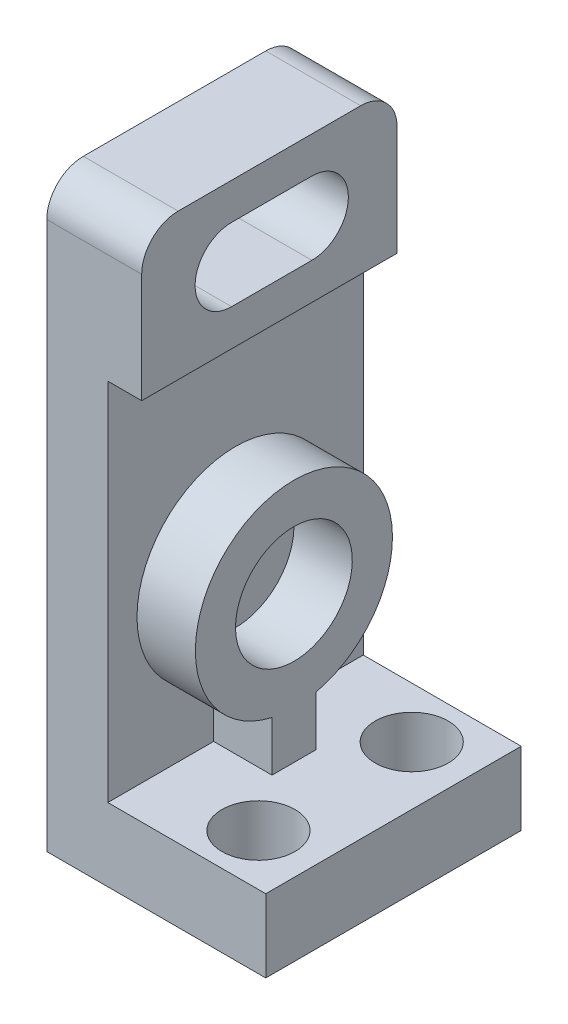
ISO-10303-21;
HEADER;
FILE_DESCRIPTION(('STEP AP214'),'2;1');
FILE_NAME('part.step','',(''),(''),'','','');
FILE_SCHEMA(('AUTOMOTIVE_DESIGN { 1 0 10303 214 1 1 1 1 }'));
ENDSEC;
DATA;
#1=APPLICATION_CONTEXT('core data for automotive mechanical design processes');
#2=APPLICATION_PROTOCOL_DEFINITION('international standard','automotive_design',2000,#1);
#3=PRODUCT_CONTEXT('',#1,'mechanical');
#4=PRODUCT('Part','Part','',(#3));
#5=PRODUCT_RELATED_PRODUCT_CATEGORY('part','',(#4));
#6=PRODUCT_DEFINITION_FORMATION('','',#4);
#7=PRODUCT_DEFINITION_CONTEXT('part definition',#1,'design');
#8=PRODUCT_DEFINITION('design','',#6,#7);
#9=PRODUCT_DEFINITION_SHAPE('','',#8);
#10=(LENGTH_UNIT() NAMED_UNIT(*) SI_UNIT(.MILLI.,.METRE.));
#11=(NAMED_UNIT(*) PLANE_ANGLE_UNIT() SI_UNIT($,.RADIAN.));
#12=(NAMED_UNIT(*) SI_UNIT($,.STERADIAN.) SOLID_ANGLE_UNIT());
#13=UNCERTAINTY_MEASURE_WITH_UNIT(LENGTH_MEASURE(1.E-05),#10,'distance_accuracy_value','');
#14=(GEOMETRIC_REPRESENTATION_CONTEXT(3) GLOBAL_UNCERTAINTY_ASSIGNED_CONTEXT((#13)) GLOBAL_UNIT_ASSIGNED_CONTEXT((#10,
#11,#12)) REPRESENTATION_CONTEXT('',''));
#15=CARTESIAN_POINT('',(0.,0.,0.));
#16=DIRECTION('',(0.,0.,1.));
#17=DIRECTION('',(1.,0.,0.));
#18=AXIS2_PLACEMENT_3D('',#15,#16,#17);
#19=CARTESIAN_POINT('',(8.35866126385831,-30.,-17.5));
#20=DIRECTION('',(0.,-1.,0.));
#21=DIRECTION('',(1.,0.,0.));
#22=AXIS2_PLACEMENT_3D('',#19,#20,#21);
#23=PLANE('',#22);
#24=CARTESIAN_POINT('',(22.,-30.,-10.5));
#25=DIRECTION('',(0.,1.,0.));
#26=DIRECTION('',(-1.,0.,0.));
#27=AXIS2_PLACEMENT_3D('',#24,#25,#26);
#28=CIRCLE('',#27,5.);
#29=CARTESIAN_POINT('',(17.,-30.,-10.5));
#30=VERTEX_POINT('',#29);
#31=EDGE_CURVE('E202',#30,#30,#28,.T.);
#32=ORIENTED_EDGE('',*,*,#31,.F.);
#33=EDGE_LOOP('',(#32));
#34=FACE_BOUND('',#33,.T.);
#35=CARTESIAN_POINT('',(22.,-30.,10.5));
#36=DIRECTION('',(0.,1.,0.));
#37=DIRECTION('',(1.,0.,0.));
#38=AXIS2_PLACEMENT_3D('',#35,#36,#37);
#39=CIRCLE('',#38,5.);
#40=CARTESIAN_POINT('',(27.,-30.,10.5));
#41=VERTEX_POINT('',#40);
#42=EDGE_CURVE('E206',#41,#41,#39,.T.);
#43=ORIENTED_EDGE('',*,*,#42,.F.);
#44=EDGE_LOOP('',(#43));
#45=FACE_BOUND('',#44,.T.);
#46=DIRECTION('',(-1.,0.,0.));
#47=VECTOR('',#46,1.);
#48=CARTESIAN_POINT('',(16.3586612638583,-30.,-3.00000000000001));
#49=LINE('',#48,#47);
#50=CARTESIAN_POINT('',(16.3586612638583,-30.,-3.00000000000001));
#51=VERTEX_POINT('',#50);
#52=CARTESIAN_POINT('',(8.35866126385831,-30.,-3.00000000000001));
#53=VERTEX_POINT('',#52);
#54=EDGE_CURVE('E229',#51,#53,#49,.T.);
#55=ORIENTED_EDGE('',*,*,#54,.F.);
#56=DIRECTION('',(0.,0.,-1.));
#57=VECTOR('',#56,1.);
#58=CARTESIAN_POINT('',(16.3586612638583,-30.,2.99999999999999));
#59=LINE('',#58,#57);
#60=CARTESIAN_POINT('',(16.3586612638583,-30.,2.99999999999999));
#61=VERTEX_POINT('',#60);
#62=EDGE_CURVE('E226',#61,#51,#59,.T.);
#63=ORIENTED_EDGE('',*,*,#62,.F.);
#64=DIRECTION('',(-1.,0.,0.));
#65=VECTOR('',#64,1.);
#66=CARTESIAN_POINT('',(16.3586612638583,-30.,2.99999999999999));
#67=LINE('',#66,#65);
#68=CARTESIAN_POINT('',(8.35866126385831,-30.,2.99999999999999));
#69=VERTEX_POINT('',#68);
#70=EDGE_CURVE('E238',#61,#69,#67,.T.);
#71=ORIENTED_EDGE('',*,*,#70,.T.);
#72=DIRECTION('',(0.,0.,1.));
#73=VECTOR('',#72,1.);
#74=CARTESIAN_POINT('',(8.35866126385831,-30.,-17.5));
#75=LINE('',#74,#73);
#76=CARTESIAN_POINT('',(8.35866126385831,-30.,17.5));
#77=VERTEX_POINT('',#76);
#78=EDGE_CURVE('E273',#69,#77,#75,.T.);
#79=ORIENTED_EDGE('',*,*,#78,.T.);
#80=DIRECTION('',(1.,0.,0.));
#81=VECTOR('',#80,1.);
#82=CARTESIAN_POINT('',(8.35866126385831,-30.,17.5));
#83=LINE('',#82,#81);
#84=CARTESIAN_POINT('',(30.,-30.,17.5));
#85=VERTEX_POINT('',#84);
#86=EDGE_CURVE('E249',#77,#85,#83,.T.);
#87=ORIENTED_EDGE('',*,*,#86,.T.);
#88=DIRECTION('',(0.,0.,1.));
#89=VECTOR('',#88,1.);
#90=CARTESIAN_POINT('',(30.,-30.,-17.5));
#91=LINE('',#90,#89);
#92=CARTESIAN_POINT('',(30.,-30.,-17.5));
#93=VERTEX_POINT('',#92);
#94=EDGE_CURVE('E270',#93,#85,#91,.T.);
#95=ORIENTED_EDGE('',*,*,#94,.F.);
#96=DIRECTION('',(1.,0.,0.));
#97=VECTOR('',#96,1.);
#98=CARTESIAN_POINT('',(8.35866126385831,-30.,-17.5));
#99=LINE('',#98,#97);
#100=CARTESIAN_POINT('',(8.35866126385831,-30.,-17.5));
#101=VERTEX_POINT('',#100);
#102=EDGE_CURVE('E257',#101,#93,#99,.T.);
#103=ORIENTED_EDGE('',*,*,#102,.F.);
#104=EDGE_CURVE('E275',#101,#53,#75,.T.);
#105=ORIENTED_EDGE('',*,*,#104,.T.);
#106=EDGE_LOOP('',(#55,#63,#71,#79,#87,#95,#103,#105));
#107=FACE_BOUND('',#106,.T.);
#108=ADVANCED_FACE('F39',(#34,#45,#107),#23,.F.);
#109=CARTESIAN_POINT('',(8.3586612638583,20.,-17.5));
#110=DIRECTION('',(-1.,0.,0.));
#111=DIRECTION('',(0.,-1.,0.));
#112=AXIS2_PLACEMENT_3D('',#109,#110,#111);
#113=PLANE('',#112);
#114=DIRECTION('',(0.,1.,0.));
#115=VECTOR('',#114,1.);
#116=CARTESIAN_POINT('',(8.35866126385831,-30.,-3.00000000000001));
#117=LINE('',#116,#115);
#118=CARTESIAN_POINT('',(8.35866126385831,-23.1624465810882,-3.00000000000001));
#119=VERTEX_POINT('',#118);
#120=EDGE_CURVE('E217',#53,#119,#117,.T.);
#121=ORIENTED_EDGE('',*,*,#120,.F.);
#122=ORIENTED_EDGE('',*,*,#104,.F.);
#123=DIRECTION('',(0.,-1.,0.));
#124=VECTOR('',#123,1.);
#125=CARTESIAN_POINT('',(8.3586612638583,20.,-17.5));
#126=LINE('',#125,#124);
#127=CARTESIAN_POINT('',(8.3586612638583,20.,-17.5));
#128=VERTEX_POINT('',#127);
#129=EDGE_CURVE('E254',#128,#101,#126,.T.);
#130=ORIENTED_EDGE('',*,*,#129,.F.);
#131=DIRECTION('',(0.,0.,1.));
#132=VECTOR('',#131,1.);
#133=CARTESIAN_POINT('',(8.3586612638583,20.,-17.5));
#134=LINE('',#133,#132);
#135=CARTESIAN_POINT('',(8.3586612638583,20.,17.5));
#136=VERTEX_POINT('',#135);
#137=EDGE_CURVE('E277',#128,#136,#134,.T.);
#138=ORIENTED_EDGE('',*,*,#137,.T.);
#139=DIRECTION('',(0.,-1.,0.));
#140=VECTOR('',#139,1.);
#141=CARTESIAN_POINT('',(8.3586612638583,20.,17.5));
#142=LINE('',#141,#140);
#143=EDGE_CURVE('E261',#136,#77,#142,.T.);
#144=ORIENTED_EDGE('',*,*,#143,.T.);
#145=ORIENTED_EDGE('',*,*,#78,.F.);
#146=DIRECTION('',(0.,1.,0.));
#147=VECTOR('',#146,1.);
#148=CARTESIAN_POINT('',(8.35866126385831,-30.,2.99999999999999));
#149=LINE('',#148,#147);
#150=CARTESIAN_POINT('',(8.35866126385831,-23.1624465810882,2.99999999999999));
#151=VERTEX_POINT('',#150);
#152=EDGE_CURVE('E225',#69,#151,#149,.T.);
#153=ORIENTED_EDGE('',*,*,#152,.T.);
#154=CARTESIAN_POINT('',(8.35866126385831,-10.,0.));
#155=DIRECTION('',(1.,0.,0.));
#156=DIRECTION('',(0.,1.,0.));
#157=AXIS2_PLACEMENT_3D('',#154,#155,#156);
#158=CIRCLE('',#157,13.5);
#159=EDGE_CURVE('E231',#119,#151,#158,.T.);
#160=ORIENTED_EDGE('',*,*,#159,.F.);
#161=EDGE_LOOP('',(#121,#122,#130,#138,#144,#145,#153,#160));
#162=FACE_BOUND('',#161,.T.);
#163=ADVANCED_FACE('F356',(#162),#113,.F.);
#164=CARTESIAN_POINT('',(30.,40.,-17.5));
#165=DIRECTION('',(0.,0.,1.));
#166=DIRECTION('',(0.,-1.,0.));
#167=AXIS2_PLACEMENT_3D('',#164,#165,#166);
#168=PLANE('',#167);
#169=DIRECTION('',(0.,1.,0.));
#170=VECTOR('',#169,1.);
#171=CARTESIAN_POINT('',(0.,40.,-17.5));
#172=LINE('',#171,#170);
#173=CARTESIAN_POINT('',(0.,-40.,-17.5));
#174=VERTEX_POINT('',#173);
#175=CARTESIAN_POINT('',(0.,35.,-17.5));
#176=VERTEX_POINT('',#175);
#177=EDGE_CURVE('E272',#174,#176,#172,.T.);
#178=ORIENTED_EDGE('',*,*,#177,.T.);
#179=DIRECTION('',(-1.,0.,0.));
#180=VECTOR('',#179,1.);
#181=CARTESIAN_POINT('',(30.,35.,-17.5));
#182=LINE('',#181,#180);
#183=CARTESIAN_POINT('',(13.,35.,-17.5));
#184=VERTEX_POINT('',#183);
#185=EDGE_CURVE('E313',#176,#184,#182,.F.);
#186=ORIENTED_EDGE('',*,*,#185,.T.);
#187=DIRECTION('',(0.,-1.,0.));
#188=VECTOR('',#187,1.);
#189=CARTESIAN_POINT('',(13.,40.,-17.5));
#190=LINE('',#189,#188);
#191=CARTESIAN_POINT('',(13.,20.,-17.5));
#192=VERTEX_POINT('',#191);
#193=EDGE_CURVE('E250',#184,#192,#190,.T.);
#194=ORIENTED_EDGE('',*,*,#193,.T.);
#195=DIRECTION('',(-1.,0.,0.));
#196=VECTOR('',#195,1.);
#197=CARTESIAN_POINT('',(13.,20.,-17.5));
#198=LINE('',#197,#196);
#199=EDGE_CURVE('E248',#192,#128,#198,.T.);
#200=ORIENTED_EDGE('',*,*,#199,.T.);
#201=ORIENTED_EDGE('',*,*,#129,.T.);
#202=ORIENTED_EDGE('',*,*,#102,.T.);
#203=DIRECTION('',(0.,1.,0.));
#204=VECTOR('',#203,1.);
#205=CARTESIAN_POINT('',(30.,40.,-17.5));
#206=LINE('',#205,#204);
#207=CARTESIAN_POINT('',(30.,-40.,-17.5));
#208=VERTEX_POINT('',#207);
#209=EDGE_CURVE('E284',#208,#93,#206,.T.);
#210=ORIENTED_EDGE('',*,*,#209,.F.);
#211=DIRECTION('',(-1.,0.,0.));
#212=VECTOR('',#211,1.);
#213=CARTESIAN_POINT('',(30.,-40.,-17.5));
#214=LINE('',#213,#212);
#215=EDGE_CURVE('E293',#208,#174,#214,.T.);
#216=ORIENTED_EDGE('',*,*,#215,.T.);
#217=EDGE_LOOP('',(#178,#186,#194,#200,#201,#202,#210,#216));
#218=FACE_BOUND('',#217,.T.);
#219=ADVANCED_FACE('F332',(#218),#168,.F.);
#220=CARTESIAN_POINT('',(30.,40.,17.5));
#221=DIRECTION('',(0.,-1.,0.));
#222=DIRECTION('',(0.,0.,-1.));
#223=AXIS2_PLACEMENT_3D('',#220,#221,#222);
#224=PLANE('',#223);
#225=DIRECTION('',(0.,0.,1.));
#226=VECTOR('',#225,1.);
#227=CARTESIAN_POINT('',(13.,40.,-17.5));
#228=LINE('',#227,#226);
#229=CARTESIAN_POINT('',(13.,40.,-12.5));
#230=VERTEX_POINT('',#229);
#231=CARTESIAN_POINT('',(13.,40.,12.5));
#232=VERTEX_POINT('',#231);
#233=EDGE_CURVE('E256',#230,#232,#228,.T.);
#234=ORIENTED_EDGE('',*,*,#233,.F.);
#235=DIRECTION('',(-1.,0.,0.));
#236=VECTOR('',#235,1.);
#237=CARTESIAN_POINT('',(30.,40.,-12.5));
#238=LINE('',#237,#236);
#239=CARTESIAN_POINT('',(0.,40.,-12.5));
#240=VERTEX_POINT('',#239);
#241=EDGE_CURVE('E310',#230,#240,#238,.T.);
#242=ORIENTED_EDGE('',*,*,#241,.T.);
#243=DIRECTION('',(0.,0.,1.));
#244=VECTOR('',#243,1.);
#245=CARTESIAN_POINT('',(0.,40.,17.5));
#246=LINE('',#245,#244);
#247=CARTESIAN_POINT('',(0.,40.,12.5));
#248=VERTEX_POINT('',#247);
#249=EDGE_CURVE('E295',#240,#248,#246,.T.);
#250=ORIENTED_EDGE('',*,*,#249,.T.);
#251=DIRECTION('',(-1.,0.,0.));
#252=VECTOR('',#251,1.);
#253=CARTESIAN_POINT('',(30.,40.,12.5));
#254=LINE('',#253,#252);
#255=EDGE_CURVE('E304',#248,#232,#254,.F.);
#256=ORIENTED_EDGE('',*,*,#255,.T.);
#257=EDGE_LOOP('',(#234,#242,#250,#256));
#258=FACE_BOUND('',#257,.T.);
#259=ADVANCED_FACE('F329',(#258),#224,.F.);
#260=CARTESIAN_POINT('',(30.,40.,17.5));
#261=DIRECTION('',(0.,0.,-1.));
#262=DIRECTION('',(0.,1.,0.));
#263=AXIS2_PLACEMENT_3D('',#260,#261,#262);
#264=PLANE('',#263);
#265=DIRECTION('',(0.,-1.,0.));
#266=VECTOR('',#265,1.);
#267=CARTESIAN_POINT('',(13.,40.,17.5));
#268=LINE('',#267,#266);
#269=CARTESIAN_POINT('',(13.,35.,17.5));
#270=VERTEX_POINT('',#269);
#271=CARTESIAN_POINT('',(13.,20.,17.5));
#272=VERTEX_POINT('',#271);
#273=EDGE_CURVE('E246',#270,#272,#268,.T.);
#274=ORIENTED_EDGE('',*,*,#273,.F.);
#275=DIRECTION('',(-1.,0.,0.));
#276=VECTOR('',#275,1.);
#277=CARTESIAN_POINT('',(30.,35.,17.5));
#278=LINE('',#277,#276);
#279=CARTESIAN_POINT('',(0.,35.,17.5));
#280=VERTEX_POINT('',#279);
#281=EDGE_CURVE('E11',#270,#280,#278,.T.);
#282=ORIENTED_EDGE('',*,*,#281,.T.);
#283=DIRECTION('',(0.,-1.,0.));
#284=VECTOR('',#283,1.);
#285=CARTESIAN_POINT('',(0.,40.,17.5));
#286=LINE('',#285,#284);
#287=CARTESIAN_POINT('',(0.,-40.,17.5));
#288=VERTEX_POINT('',#287);
#289=EDGE_CURVE('E300',#280,#288,#286,.T.);
#290=ORIENTED_EDGE('',*,*,#289,.T.);
#291=DIRECTION('',(-1.,0.,0.));
#292=VECTOR('',#291,1.);
#293=CARTESIAN_POINT('',(30.,-40.,17.5));
#294=LINE('',#293,#292);
#295=CARTESIAN_POINT('',(30.,-40.,17.5));
#296=VERTEX_POINT('',#295);
#297=EDGE_CURVE('E305',#296,#288,#294,.T.);
#298=ORIENTED_EDGE('',*,*,#297,.F.);
#299=DIRECTION('',(0.,-1.,0.));
#300=VECTOR('',#299,1.);
#301=CARTESIAN_POINT('',(30.,40.,17.5));
#302=LINE('',#301,#300);
#303=EDGE_CURVE('E289',#85,#296,#302,.T.);
#304=ORIENTED_EDGE('',*,*,#303,.F.);
#305=ORIENTED_EDGE('',*,*,#86,.F.);
#306=ORIENTED_EDGE('',*,*,#143,.F.);
#307=DIRECTION('',(-1.,0.,0.));
#308=VECTOR('',#307,1.);
#309=CARTESIAN_POINT('',(13.,20.,17.5));
#310=LINE('',#309,#308);
#311=EDGE_CURVE('E262',#272,#136,#310,.T.);
#312=ORIENTED_EDGE('',*,*,#311,.F.);
#313=EDGE_LOOP('',(#274,#282,#290,#298,#304,#305,#306,#312));
#314=FACE_BOUND('',#313,.T.);
#315=ADVANCED_FACE('F343',(#314),#264,.F.);
#316=CARTESIAN_POINT('',(30.,-40.,17.5));
#317=DIRECTION('',(0.,1.,0.));
#318=DIRECTION('',(0.,0.,1.));
#319=AXIS2_PLACEMENT_3D('',#316,#317,#318);
#320=PLANE('',#319);
#321=CARTESIAN_POINT('',(22.,-40.,-10.5));
#322=DIRECTION('',(0.,1.,0.));
#323=DIRECTION('',(-1.,0.,0.));
#324=AXIS2_PLACEMENT_3D('',#321,#322,#323);
#325=CIRCLE('',#324,5.);
#326=CARTESIAN_POINT('',(17.,-40.,-10.5));
#327=VERTEX_POINT('',#326);
#328=EDGE_CURVE('E204',#327,#327,#325,.T.);
#329=ORIENTED_EDGE('',*,*,#328,.T.);
#330=EDGE_LOOP('',(#329));
#331=FACE_BOUND('',#330,.T.);
#332=CARTESIAN_POINT('',(22.,-40.,10.5));
#333=DIRECTION('',(0.,1.,0.));
#334=DIRECTION('',(1.,0.,0.));
#335=AXIS2_PLACEMENT_3D('',#332,#333,#334);
#336=CIRCLE('',#335,5.);
#337=CARTESIAN_POINT('',(27.,-40.,10.5));
#338=VERTEX_POINT('',#337);
#339=EDGE_CURVE('E200',#338,#338,#336,.T.);
#340=ORIENTED_EDGE('',*,*,#339,.T.);
#341=EDGE_LOOP('',(#340));
#342=FACE_BOUND('',#341,.T.);
#343=DIRECTION('',(0.,0.,-1.));
#344=VECTOR('',#343,1.);
#345=CARTESIAN_POINT('',(0.,-40.,17.5));
#346=LINE('',#345,#344);
#347=EDGE_CURVE('E286',#288,#174,#346,.T.);
#348=ORIENTED_EDGE('',*,*,#347,.T.);
#349=ORIENTED_EDGE('',*,*,#215,.F.);
#350=DIRECTION('',(0.,0.,-1.));
#351=VECTOR('',#350,1.);
#352=CARTESIAN_POINT('',(30.,-40.,17.5));
#353=LINE('',#352,#351);
#354=EDGE_CURVE('E288',#296,#208,#353,.T.);
#355=ORIENTED_EDGE('',*,*,#354,.F.);
#356=ORIENTED_EDGE('',*,*,#297,.T.);
#357=EDGE_LOOP('',(#348,#349,#355,#356));
#358=FACE_BOUND('',#357,.T.);
#359=ADVANCED_FACE('F338',(#331,#342,#358),#320,.F.);
#360=CARTESIAN_POINT('',(30.,0.,0.));
#361=DIRECTION('',(1.,0.,0.));
#362=DIRECTION('',(0.,0.,-1.));
#363=AXIS2_PLACEMENT_3D('',#360,#361,#362);
#364=PLANE('',#363);
#365=ORIENTED_EDGE('',*,*,#94,.T.);
#366=ORIENTED_EDGE('',*,*,#303,.T.);
#367=ORIENTED_EDGE('',*,*,#354,.T.);
#368=ORIENTED_EDGE('',*,*,#209,.T.);
#369=EDGE_LOOP('',(#365,#366,#367,#368));
#370=FACE_BOUND('',#369,.T.);
#371=ADVANCED_FACE('F361',(#370),#364,.T.);
#372=CARTESIAN_POINT('',(0.,0.,0.));
#373=DIRECTION('',(1.,0.,0.));
#374=DIRECTION('',(0.,0.,-1.));
#375=AXIS2_PLACEMENT_3D('',#372,#373,#374);
#376=PLANE('',#375);
#377=DIRECTION('',(0.,0.,1.));
#378=VECTOR('',#377,1.);
#379=CARTESIAN_POINT('',(0.,35.,5.18095085404985));
#380=LINE('',#379,#378);
#381=CARTESIAN_POINT('',(0.,35.,-5.81904914595015));
#382=VERTEX_POINT('',#381);
#383=CARTESIAN_POINT('',(0.,35.,5.18095085404985));
#384=VERTEX_POINT('',#383);
#385=EDGE_CURVE('E175',#382,#384,#380,.T.);
#386=ORIENTED_EDGE('',*,*,#385,.T.);
#387=CARTESIAN_POINT('',(0.,30.,5.18095085404985));
#388=DIRECTION('',(1.,0.,0.));
#389=DIRECTION('',(0.,1.,0.));
#390=AXIS2_PLACEMENT_3D('',#387,#388,#389);
#391=CIRCLE('',#390,5.);
#392=CARTESIAN_POINT('',(0.,25.,5.18095085404985));
#393=VERTEX_POINT('',#392);
#394=EDGE_CURVE('E168',#384,#393,#391,.T.);
#395=ORIENTED_EDGE('',*,*,#394,.T.);
#396=DIRECTION('',(0.,0.,-1.));
#397=VECTOR('',#396,1.);
#398=CARTESIAN_POINT('',(0.,25.,5.18095085404985));
#399=LINE('',#398,#397);
#400=CARTESIAN_POINT('',(0.,25.,-5.81904914595015));
#401=VERTEX_POINT('',#400);
#402=EDGE_CURVE('E174',#393,#401,#399,.T.);
#403=ORIENTED_EDGE('',*,*,#402,.T.);
#404=CARTESIAN_POINT('',(0.,30.,-5.81904914595015));
#405=DIRECTION('',(1.,0.,0.));
#406=DIRECTION('',(0.,1.,0.));
#407=AXIS2_PLACEMENT_3D('',#404,#405,#406);
#408=CIRCLE('',#407,5.);
#409=EDGE_CURVE('E53',#401,#382,#408,.T.);
#410=ORIENTED_EDGE('',*,*,#409,.T.);
#411=EDGE_LOOP('',(#386,#395,#403,#410));
#412=FACE_BOUND('',#411,.T.);
#413=ORIENTED_EDGE('',*,*,#249,.F.);
#414=CARTESIAN_POINT('',(0.,35.,-12.5));
#415=DIRECTION('',(1.,0.,0.));
#416=DIRECTION('',(0.,0.,-1.));
#417=AXIS2_PLACEMENT_3D('',#414,#415,#416);
#418=CIRCLE('',#417,5.);
#419=EDGE_CURVE('E315',#240,#176,#418,.F.);
#420=ORIENTED_EDGE('',*,*,#419,.T.);
#421=ORIENTED_EDGE('',*,*,#177,.F.);
#422=ORIENTED_EDGE('',*,*,#347,.F.);
#423=ORIENTED_EDGE('',*,*,#289,.F.);
#424=CARTESIAN_POINT('',(0.,35.,12.5));
#425=DIRECTION('',(1.,0.,0.));
#426=DIRECTION('',(0.,0.,-1.));
#427=AXIS2_PLACEMENT_3D('',#424,#425,#426);
#428=CIRCLE('',#427,5.);
#429=EDGE_CURVE('E309',#280,#248,#428,.F.);
#430=ORIENTED_EDGE('',*,*,#429,.T.);
#431=EDGE_LOOP('',(#413,#420,#421,#422,#423,#430));
#432=FACE_BOUND('',#431,.T.);
#433=ADVANCED_FACE('F177',(#412,#432),#376,.F.);
#434=CARTESIAN_POINT('',(13.,20.,-17.5));
#435=DIRECTION('',(0.,1.,0.));
#436=DIRECTION('',(0.,0.,1.));
#437=AXIS2_PLACEMENT_3D('',#434,#435,#436);
#438=PLANE('',#437);
#439=ORIENTED_EDGE('',*,*,#311,.T.);
#440=ORIENTED_EDGE('',*,*,#137,.F.);
#441=ORIENTED_EDGE('',*,*,#199,.F.);
#442=DIRECTION('',(0.,0.,1.));
#443=VECTOR('',#442,1.);
#444=CARTESIAN_POINT('',(13.,20.,-17.5));
#445=LINE('',#444,#443);
#446=EDGE_CURVE('E279',#192,#272,#445,.T.);
#447=ORIENTED_EDGE('',*,*,#446,.T.);
#448=EDGE_LOOP('',(#439,#440,#441,#447));
#449=FACE_BOUND('',#448,.T.);
#450=ADVANCED_FACE('F351',(#449),#438,.F.);
#451=CARTESIAN_POINT('',(13.,40.,-17.5));
#452=DIRECTION('',(-1.,0.,0.));
#453=DIRECTION('',(0.,-1.,0.));
#454=AXIS2_PLACEMENT_3D('',#451,#452,#453);
#455=PLANE('',#454);
#456=DIRECTION('',(0.,0.,-1.));
#457=VECTOR('',#456,1.);
#458=CARTESIAN_POINT('',(13.,25.,5.18095085404985));
#459=LINE('',#458,#457);
#460=CARTESIAN_POINT('',(13.,25.,5.18095085404985));
#461=VERTEX_POINT('',#460);
#462=CARTESIAN_POINT('',(13.,25.,-5.81904914595015));
#463=VERTEX_POINT('',#462);
#464=EDGE_CURVE('E192',#461,#463,#459,.T.);
#465=ORIENTED_EDGE('',*,*,#464,.F.);
#466=CARTESIAN_POINT('',(13.,30.,5.18095085404985));
#467=DIRECTION('',(1.,0.,0.));
#468=DIRECTION('',(0.,1.,0.));
#469=AXIS2_PLACEMENT_3D('',#466,#467,#468);
#470=CIRCLE('',#469,5.);
#471=CARTESIAN_POINT('',(13.,35.,5.18095085404985));
#472=VERTEX_POINT('',#471);
#473=EDGE_CURVE('E65',#472,#461,#470,.T.);
#474=ORIENTED_EDGE('',*,*,#473,.F.);
#475=DIRECTION('',(0.,0.,1.));
#476=VECTOR('',#475,1.);
#477=CARTESIAN_POINT('',(13.,35.,5.18095085404985));
#478=LINE('',#477,#476);
#479=CARTESIAN_POINT('',(13.,35.,-5.81904914595015));
#480=VERTEX_POINT('',#479);
#481=EDGE_CURVE('E185',#480,#472,#478,.T.);
#482=ORIENTED_EDGE('',*,*,#481,.F.);
#483=CARTESIAN_POINT('',(13.,30.,-5.81904914595015));
#484=DIRECTION('',(1.,0.,0.));
#485=DIRECTION('',(0.,1.,0.));
#486=AXIS2_PLACEMENT_3D('',#483,#484,#485);
#487=CIRCLE('',#486,5.);
#488=EDGE_CURVE('E184',#463,#480,#487,.T.);
#489=ORIENTED_EDGE('',*,*,#488,.F.);
#490=EDGE_LOOP('',(#465,#474,#482,#489));
#491=FACE_BOUND('',#490,.T.);
#492=ORIENTED_EDGE('',*,*,#193,.F.);
#493=CARTESIAN_POINT('',(13.,35.,-12.5));
#494=DIRECTION('',(-1.,0.,0.));
#495=DIRECTION('',(0.,-1.,0.));
#496=AXIS2_PLACEMENT_3D('',#493,#494,#495);
#497=CIRCLE('',#496,5.);
#498=EDGE_CURVE('E50',#184,#230,#497,.F.);
#499=ORIENTED_EDGE('',*,*,#498,.T.);
#500=ORIENTED_EDGE('',*,*,#233,.T.);
#501=CARTESIAN_POINT('',(13.,35.,12.5));
#502=DIRECTION('',(-1.,0.,0.));
#503=DIRECTION('',(0.,-1.,0.));
#504=AXIS2_PLACEMENT_3D('',#501,#502,#503);
#505=CIRCLE('',#504,5.);
#506=EDGE_CURVE('E317',#232,#270,#505,.F.);
#507=ORIENTED_EDGE('',*,*,#506,.T.);
#508=ORIENTED_EDGE('',*,*,#273,.T.);
#509=ORIENTED_EDGE('',*,*,#446,.F.);
#510=EDGE_LOOP('',(#492,#499,#500,#507,#508,#509));
#511=FACE_BOUND('',#510,.T.);
#512=ADVANCED_FACE('F322',(#491,#511),#455,.F.);
#513=CARTESIAN_POINT('',(16.3586612638583,-30.,-3.00000000000001));
#514=DIRECTION('',(0.,0.,1.));
#515=DIRECTION('',(1.,0.,0.));
#516=AXIS2_PLACEMENT_3D('',#513,#514,#515);
#517=PLANE('',#516);
#518=ORIENTED_EDGE('',*,*,#120,.T.);
#519=DIRECTION('',(-1.,0.,0.));
#520=VECTOR('',#519,1.);
#521=CARTESIAN_POINT('',(16.3586612638583,-23.1624465810882,-3.00000000000001));
#522=LINE('',#521,#520);
#523=CARTESIAN_POINT('',(16.3586612638583,-23.1624465810882,-3.00000000000001));
#524=VERTEX_POINT('',#523);
#525=EDGE_CURVE('E242',#524,#119,#522,.T.);
#526=ORIENTED_EDGE('',*,*,#525,.F.);
#527=DIRECTION('',(0.,1.,0.));
#528=VECTOR('',#527,1.);
#529=CARTESIAN_POINT('',(16.3586612638583,-30.,-3.00000000000001));
#530=LINE('',#529,#528);
#531=EDGE_CURVE('E216',#51,#524,#530,.T.);
#532=ORIENTED_EDGE('',*,*,#531,.F.);
#533=ORIENTED_EDGE('',*,*,#54,.T.);
#534=EDGE_LOOP('',(#518,#526,#532,#533));
#535=FACE_BOUND('',#534,.T.);
#536=ADVANCED_FACE('F377',(#535),#517,.F.);
#537=CARTESIAN_POINT('',(16.3586612638583,-10.,0.));
#538=DIRECTION('',(-1.,0.,0.));
#539=DIRECTION('',(0.,-1.,0.));
#540=AXIS2_PLACEMENT_3D('',#537,#538,#539);
#541=CYLINDRICAL_SURFACE('',#540,13.5);
#542=ORIENTED_EDGE('',*,*,#159,.T.);
#543=DIRECTION('',(-1.,0.,0.));
#544=VECTOR('',#543,1.);
#545=CARTESIAN_POINT('',(16.3586612638583,-23.1624465810882,2.99999999999998));
#546=LINE('',#545,#544);
#547=CARTESIAN_POINT('',(16.3586612638583,-23.1624465810882,2.99999999999998));
#548=VERTEX_POINT('',#547);
#549=EDGE_CURVE('E241',#548,#151,#546,.T.);
#550=ORIENTED_EDGE('',*,*,#549,.F.);
#551=CARTESIAN_POINT('',(16.3586612638583,-10.,0.));
#552=DIRECTION('',(1.,0.,0.));
#553=DIRECTION('',(0.,1.,0.));
#554=AXIS2_PLACEMENT_3D('',#551,#552,#553);
#555=CIRCLE('',#554,13.5);
#556=EDGE_CURVE('E221',#524,#548,#555,.T.);
#557=ORIENTED_EDGE('',*,*,#556,.F.);
#558=ORIENTED_EDGE('',*,*,#525,.T.);
#559=EDGE_LOOP('',(#542,#550,#557,#558));
#560=FACE_BOUND('',#559,.T.);
#561=ADVANCED_FACE('F374',(#560),#541,.T.);
#562=CARTESIAN_POINT('',(16.3586612638583,-30.,2.99999999999999));
#563=DIRECTION('',(0.,0.,1.));
#564=DIRECTION('',(1.,0.,0.));
#565=AXIS2_PLACEMENT_3D('',#562,#563,#564);
#566=PLANE('',#565);
#567=ORIENTED_EDGE('',*,*,#152,.F.);
#568=ORIENTED_EDGE('',*,*,#70,.F.);
#569=DIRECTION('',(0.,1.,0.));
#570=VECTOR('',#569,1.);
#571=CARTESIAN_POINT('',(16.3586612638583,-30.,2.99999999999999));
#572=LINE('',#571,#570);
#573=EDGE_CURVE('E222',#61,#548,#572,.T.);
#574=ORIENTED_EDGE('',*,*,#573,.T.);
#575=ORIENTED_EDGE('',*,*,#549,.T.);
#576=EDGE_LOOP('',(#567,#568,#574,#575));
#577=FACE_BOUND('',#576,.T.);
#578=ADVANCED_FACE('F368',(#577),#566,.T.);
#579=CARTESIAN_POINT('',(16.3586612638583,-10.,0.));
#580=DIRECTION('',(1.,0.,0.));
#581=DIRECTION('',(0.,1.,0.));
#582=AXIS2_PLACEMENT_3D('',#579,#580,#581);
#583=PLANE('',#582);
#584=CARTESIAN_POINT('',(16.3586612638583,-10.,0.));
#585=DIRECTION('',(1.,0.,0.));
#586=DIRECTION('',(0.,1.,0.));
#587=AXIS2_PLACEMENT_3D('',#584,#585,#586);
#588=CIRCLE('',#587,8.);
#589=CARTESIAN_POINT('',(16.3586612638583,-2.00000000000002,0.));
#590=VERTEX_POINT('',#589);
#591=EDGE_CURVE('E203',#590,#590,#588,.T.);
#592=ORIENTED_EDGE('',*,*,#591,.F.);
#593=EDGE_LOOP('',(#592));
#594=FACE_BOUND('',#593,.T.);
#595=ORIENTED_EDGE('',*,*,#531,.T.);
#596=ORIENTED_EDGE('',*,*,#556,.T.);
#597=ORIENTED_EDGE('',*,*,#573,.F.);
#598=ORIENTED_EDGE('',*,*,#62,.T.);
#599=EDGE_LOOP('',(#595,#596,#597,#598));
#600=FACE_BOUND('',#599,.T.);
#601=ADVANCED_FACE('F369',(#594,#600),#583,.T.);
#602=CARTESIAN_POINT('',(8.35866126385831,-10.,0.));
#603=DIRECTION('',(1.,0.,0.));
#604=DIRECTION('',(0.,1.,0.));
#605=AXIS2_PLACEMENT_3D('',#602,#603,#604);
#606=CYLINDRICAL_SURFACE('',#605,8.);
#607=CARTESIAN_POINT('',(8.35866126385831,-10.,0.));
#608=DIRECTION('',(1.,0.,0.));
#609=DIRECTION('',(0.,1.,0.));
#610=AXIS2_PLACEMENT_3D('',#607,#608,#609);
#611=CIRCLE('',#610,8.);
#612=CARTESIAN_POINT('',(8.35866126385831,-2.00000000000002,0.));
#613=VERTEX_POINT('',#612);
#614=EDGE_CURVE('E214',#613,#613,#611,.T.);
#615=ORIENTED_EDGE('',*,*,#614,.F.);
#616=EDGE_LOOP('',(#615));
#617=FACE_BOUND('',#616,.T.);
#618=ORIENTED_EDGE('',*,*,#591,.T.);
#619=EDGE_LOOP('',(#618));
#620=FACE_BOUND('',#619,.T.);
#621=ADVANCED_FACE('F432',(#617,#620),#606,.F.);
#622=CARTESIAN_POINT('',(8.35866126385831,-10.,0.));
#623=DIRECTION('',(1.,0.,0.));
#624=DIRECTION('',(0.,1.,0.));
#625=AXIS2_PLACEMENT_3D('',#622,#623,#624);
#626=PLANE('',#625);
#627=ORIENTED_EDGE('',*,*,#614,.T.);
#628=EDGE_LOOP('',(#627));
#629=FACE_BOUND('',#628,.T.);
#630=ADVANCED_FACE('F424',(#629),#626,.T.);
#631=CARTESIAN_POINT('',(22.,-40.,10.5));
#632=DIRECTION('',(0.,1.,0.));
#633=DIRECTION('',(-1.,0.,0.));
#634=AXIS2_PLACEMENT_3D('',#631,#632,#633);
#635=CYLINDRICAL_SURFACE('',#634,5.);
#636=ORIENTED_EDGE('',*,*,#339,.F.);
#637=EDGE_LOOP('',(#636));
#638=FACE_BOUND('',#637,.T.);
#639=ORIENTED_EDGE('',*,*,#42,.T.);
#640=EDGE_LOOP('',(#639));
#641=FACE_BOUND('',#640,.T.);
#642=ADVANCED_FACE('F418',(#638,#641),#635,.F.);
#643=CARTESIAN_POINT('',(22.,-40.,-10.5));
#644=DIRECTION('',(0.,1.,0.));
#645=DIRECTION('',(-1.,0.,0.));
#646=AXIS2_PLACEMENT_3D('',#643,#644,#645);
#647=CYLINDRICAL_SURFACE('',#646,5.);
#648=ORIENTED_EDGE('',*,*,#328,.F.);
#649=EDGE_LOOP('',(#648));
#650=FACE_BOUND('',#649,.T.);
#651=ORIENTED_EDGE('',*,*,#31,.T.);
#652=EDGE_LOOP('',(#651));
#653=FACE_BOUND('',#652,.T.);
#654=ADVANCED_FACE('F411',(#650,#653),#647,.F.);
#655=CARTESIAN_POINT('',(30.,35.,-12.5));
#656=DIRECTION('',(-1.,0.,0.));
#657=DIRECTION('',(0.,0.,1.));
#658=AXIS2_PLACEMENT_3D('',#655,#656,#657);
#659=CYLINDRICAL_SURFACE('',#658,5.);
#660=ORIENTED_EDGE('',*,*,#498,.F.);
#661=ORIENTED_EDGE('',*,*,#185,.F.);
#662=ORIENTED_EDGE('',*,*,#419,.F.);
#663=ORIENTED_EDGE('',*,*,#241,.F.);
#664=EDGE_LOOP('',(#660,#661,#662,#663));
#665=FACE_BOUND('',#664,.T.);
#666=ADVANCED_FACE('F334',(#665),#659,.T.);
#667=CARTESIAN_POINT('',(30.,35.,12.5));
#668=DIRECTION('',(-1.,0.,0.));
#669=DIRECTION('',(0.,0.,1.));
#670=AXIS2_PLACEMENT_3D('',#667,#668,#669);
#671=CYLINDRICAL_SURFACE('',#670,5.);
#672=ORIENTED_EDGE('',*,*,#506,.F.);
#673=ORIENTED_EDGE('',*,*,#255,.F.);
#674=ORIENTED_EDGE('',*,*,#429,.F.);
#675=ORIENTED_EDGE('',*,*,#281,.F.);
#676=EDGE_LOOP('',(#672,#673,#674,#675));
#677=FACE_BOUND('',#676,.T.);
#678=ADVANCED_FACE('F41',(#677),#671,.T.);
#679=CARTESIAN_POINT('',(0.,30.,5.18095085404985));
#680=DIRECTION('',(1.,0.,0.));
#681=DIRECTION('',(0.,1.,0.));
#682=AXIS2_PLACEMENT_3D('',#679,#680,#681);
#683=CYLINDRICAL_SURFACE('',#682,5.);
#684=ORIENTED_EDGE('',*,*,#473,.T.);
#685=DIRECTION('',(1.,0.,0.));
#686=VECTOR('',#685,1.);
#687=CARTESIAN_POINT('',(0.,25.,5.18095085404985));
#688=LINE('',#687,#686);
#689=EDGE_CURVE('E162',#393,#461,#688,.T.);
#690=ORIENTED_EDGE('',*,*,#689,.F.);
#691=ORIENTED_EDGE('',*,*,#394,.F.);
#692=DIRECTION('',(1.,0.,0.));
#693=VECTOR('',#692,1.);
#694=CARTESIAN_POINT('',(0.,35.,5.18095085404985));
#695=LINE('',#694,#693);
#696=EDGE_CURVE('E193',#384,#472,#695,.T.);
#697=ORIENTED_EDGE('',*,*,#696,.T.);
#698=EDGE_LOOP('',(#684,#690,#691,#697));
#699=FACE_BOUND('',#698,.T.);
#700=ADVANCED_FACE('F165',(#699),#683,.F.);
#701=CARTESIAN_POINT('',(0.,35.,5.18095085404985));
#702=DIRECTION('',(0.,1.,0.));
#703=DIRECTION('',(-1.,0.,0.));
#704=AXIS2_PLACEMENT_3D('',#701,#702,#703);
#705=PLANE('',#704);
#706=ORIENTED_EDGE('',*,*,#481,.T.);
#707=ORIENTED_EDGE('',*,*,#696,.F.);
#708=ORIENTED_EDGE('',*,*,#385,.F.);
#709=DIRECTION('',(1.,0.,0.));
#710=VECTOR('',#709,1.);
#711=CARTESIAN_POINT('',(0.,35.,-5.81904914595015));
#712=LINE('',#711,#710);
#713=EDGE_CURVE('E199',#382,#480,#712,.T.);
#714=ORIENTED_EDGE('',*,*,#713,.T.);
#715=EDGE_LOOP('',(#706,#707,#708,#714));
#716=FACE_BOUND('',#715,.T.);
#717=ADVANCED_FACE('F495',(#716),#705,.F.);
#718=CARTESIAN_POINT('',(0.,30.,-5.81904914595015));
#719=DIRECTION('',(1.,0.,0.));
#720=DIRECTION('',(0.,1.,0.));
#721=AXIS2_PLACEMENT_3D('',#718,#719,#720);
#722=CYLINDRICAL_SURFACE('',#721,5.);
#723=ORIENTED_EDGE('',*,*,#488,.T.);
#724=ORIENTED_EDGE('',*,*,#713,.F.);
#725=ORIENTED_EDGE('',*,*,#409,.F.);
#726=DIRECTION('',(1.,0.,0.));
#727=VECTOR('',#726,1.);
#728=CARTESIAN_POINT('',(0.,25.,-5.81904914595015));
#729=LINE('',#728,#727);
#730=EDGE_CURVE('E171',#401,#463,#729,.T.);
#731=ORIENTED_EDGE('',*,*,#730,.T.);
#732=EDGE_LOOP('',(#723,#724,#725,#731));
#733=FACE_BOUND('',#732,.T.);
#734=ADVANCED_FACE('F499',(#733),#722,.F.);
#735=CARTESIAN_POINT('',(0.,25.,5.18095085404985));
#736=DIRECTION('',(0.,-1.,0.));
#737=DIRECTION('',(1.,0.,0.));
#738=AXIS2_PLACEMENT_3D('',#735,#736,#737);
#739=PLANE('',#738);
#740=ORIENTED_EDGE('',*,*,#464,.T.);
#741=ORIENTED_EDGE('',*,*,#730,.F.);
#742=ORIENTED_EDGE('',*,*,#402,.F.);
#743=ORIENTED_EDGE('',*,*,#689,.T.);
#744=EDGE_LOOP('',(#740,#741,#742,#743));
#745=FACE_BOUND('',#744,.T.);
#746=ADVANCED_FACE('F176',(#745),#739,.F.);
#747=CLOSED_SHELL('',(#108,#163,#219,#259,#315,#359,#371,#433,#450,#512,#536,#561,#578,#601,
#621,#630,#642,#654,#666,#678,#700,#717,#734,#746));
#748=MANIFOLD_SOLID_BREP('B2',#747);
#749=ADVANCED_BREP_SHAPE_REPRESENTATION('',(#18,#748),#14);
#750=SHAPE_DEFINITION_REPRESENTATION(#9,#749);
ENDSEC;
END-ISO-10303-21;
